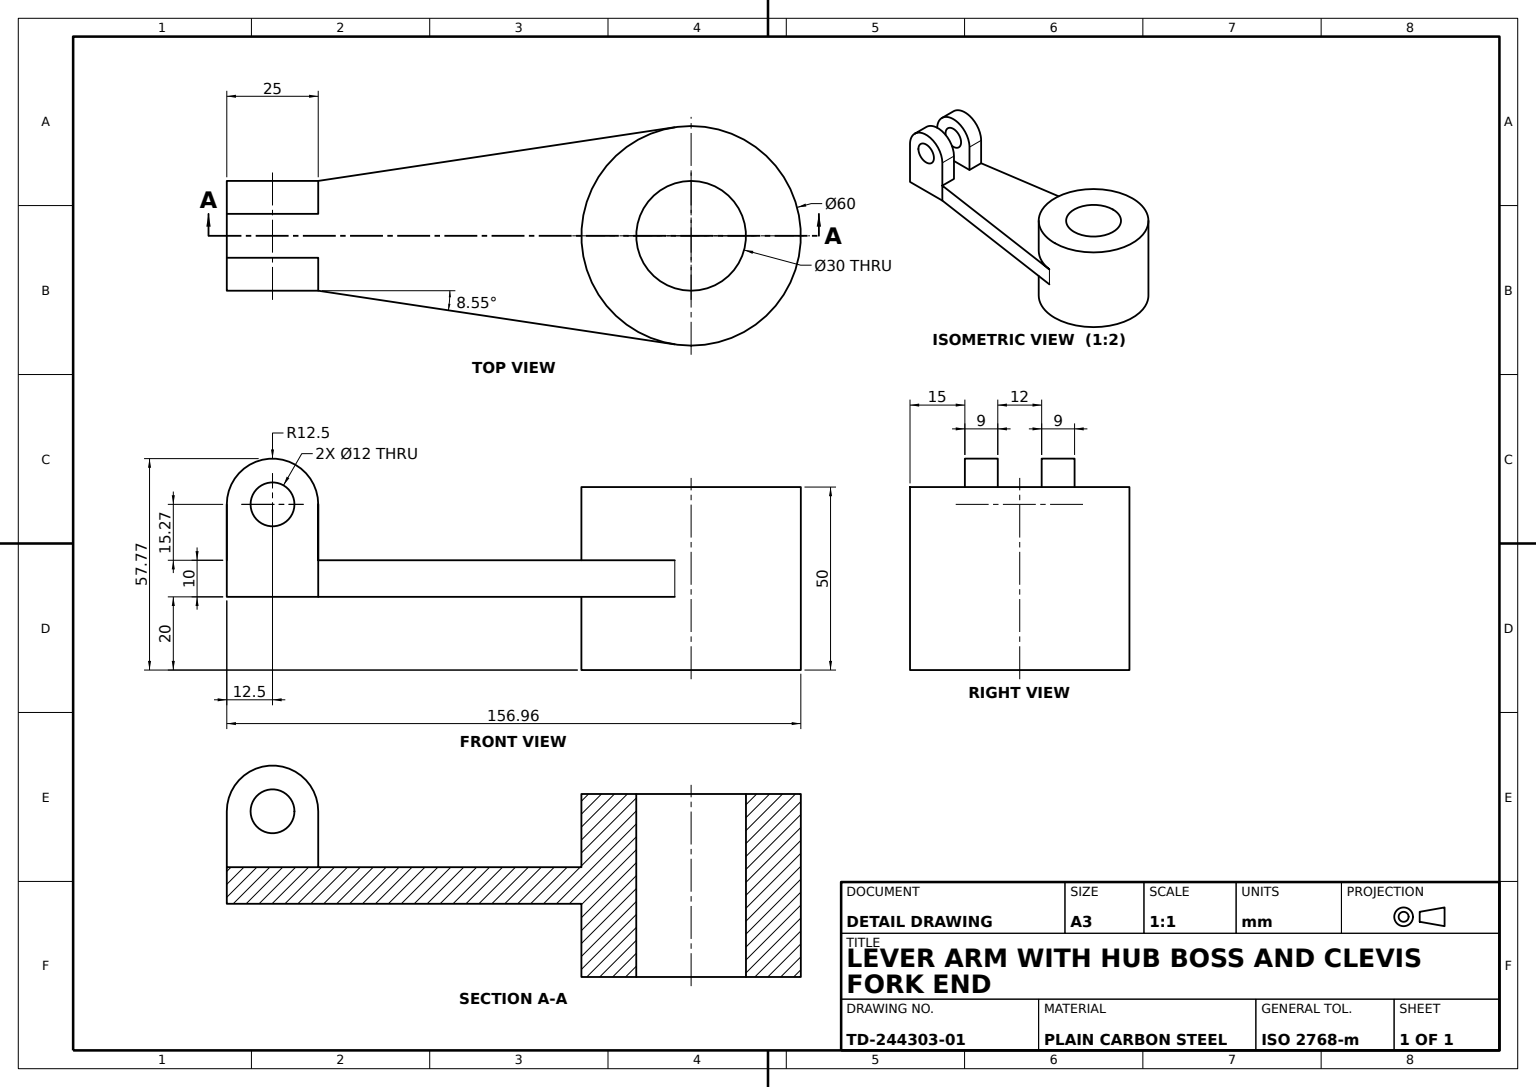
from build123d import *

# Parameters (mm, degrees)
HUB_SKETCH_60_R       = 30
HUB_60X50_DEPTH       = 25
BORE_SKETCH_30_R      = 15
HUB_BORE_30_DEPTH     = 66.574385243
ARM_PLATE_10MM_DEPTH  = 5
CLEVIS_BASE_DEPTH     = 10
CLEVIS_LUG_1_SKETCH_R = 6
CLEVIS_LUG_1_DEPTH    = 9
CLEVIS_START          = -9
CLEVIS_LUG_2_SKETCH_R = 6
CLEVIS_LUG_2_DEPTH    = 9


with BuildPart() as part:
    # Hub Sketch Ø60 → Hub Ø60x50 (new, symmetric)
    with BuildSketch(Plane(origin=(0, 0, 0), x_dir=(1, 0, 0), z_dir=(0, 1, 0))):
        with Locations(Location((0, 0, 0), (0, 0, 270))):
            Circle(HUB_SKETCH_60_R)
    extrude(amount=HUB_60X50_DEPTH, both=True)

    # Bore Sketch Ø30 → Hub Bore Ø30 (cut, through all)
    with BuildSketch(Plane(origin=(0, 25, 0), x_dir=(1, 0, 0), z_dir=(0, 1, 0))):
        with Locations(Location((0, 0, 0), (0, 0, 270))):
            Circle(BORE_SKETCH_30_R)
    extrude(amount=-HUB_BORE_30_DEPTH, mode=Mode.SUBTRACT)

    # Arm Plate Sketch → Arm Plate 10mm (add, symmetric)
    with BuildSketch(Plane(origin=(0, 0, 0), x_dir=(1, 0, 0), z_dir=(0, 1, 0))):
        with BuildLine():
            Line((-101.962487217, 15), (-4.462487217, 29.666246946))
            ThreePointArc((-4.462487217, 29.666246946), (-30, 0), (-4.462487217, -29.666246946))
            Line((-4.462487217, -29.666246946), (-101.962487217, -15))
            Line((-101.962487217, -15), (-101.962487217, 15))
        make_face()
    extrude(amount=ARM_PLATE_10MM_DEPTH, both=True)

    # Clevis Base Sketch → Clevis Base (add)
    with BuildSketch(Plane(origin=(0, 5, 0), x_dir=(1, 0, 0), z_dir=(0, 1, 0))):
        with BuildLine():
            Line((-101.962487217, -15), (-126.962487217, -15))
            Line((-126.962487217, -15), (-126.962487217, 15))
            Line((-126.962487217, 15), (-101.962487217, 15))
            Line((-101.962487217, 15), (-4.462487217, 29.666246946))
            ThreePointArc((-4.462487217, 29.666246946), (-30, 0), (-4.462487217, -29.666246946))
            Line((-4.462487217, -29.666246946), (-101.962487217, -15))
        make_face()
    extrude(amount=-CLEVIS_BASE_DEPTH)

    # Clevis Lug 1 Sketch → Clevis Lug 1 (add)
    with BuildSketch(Plane.XY.offset(15)):
        with BuildLine():
            Line((-101.962487217, 5), (-101.962487217, 20.272052395))
            ThreePointArc((-101.962487217, 20.272052395), (-114.462487217, 32.772052395), (-126.962487217, 20.272052395))
            Line((-126.962487217, 20.272052395), (-126.962487217, 5))
            Line((-126.962487217, 5), (-101.962487217, 5))
        make_face()
        with Locations((-114.462487217, 20.272052395)):
            Circle(CLEVIS_LUG_1_SKETCH_R, mode=Mode.SUBTRACT)
    extrude(amount=-CLEVIS_LUG_1_DEPTH)

    # Clevis Lug 2 Sketch → Clevis Lug 2 (add)
    with BuildSketch(Plane(origin=(0, 0, -15), x_dir=(-1, 0, 0), z_dir=(0, 0, -1)).offset(CLEVIS_START)):
        with BuildLine():
            Line((126.962487217, 20.272052395), (126.962487217, 5))
            Line((126.962487217, 5), (101.962487217, 5))
            Line((101.962487217, 5), (101.962487217, 20.272052395))
            ThreePointArc((101.962487217, 20.272052395), (114.462487217, 32.772052395), (126.962487217, 20.272052395))
        make_face()
        with Locations(Location((114.462487217, 20.272052395, 0), (0, 0, 180))):
            Circle(CLEVIS_LUG_2_SKETCH_R, mode=Mode.SUBTRACT)
    extrude(amount=CLEVIS_LUG_2_DEPTH)


solid = part.part
